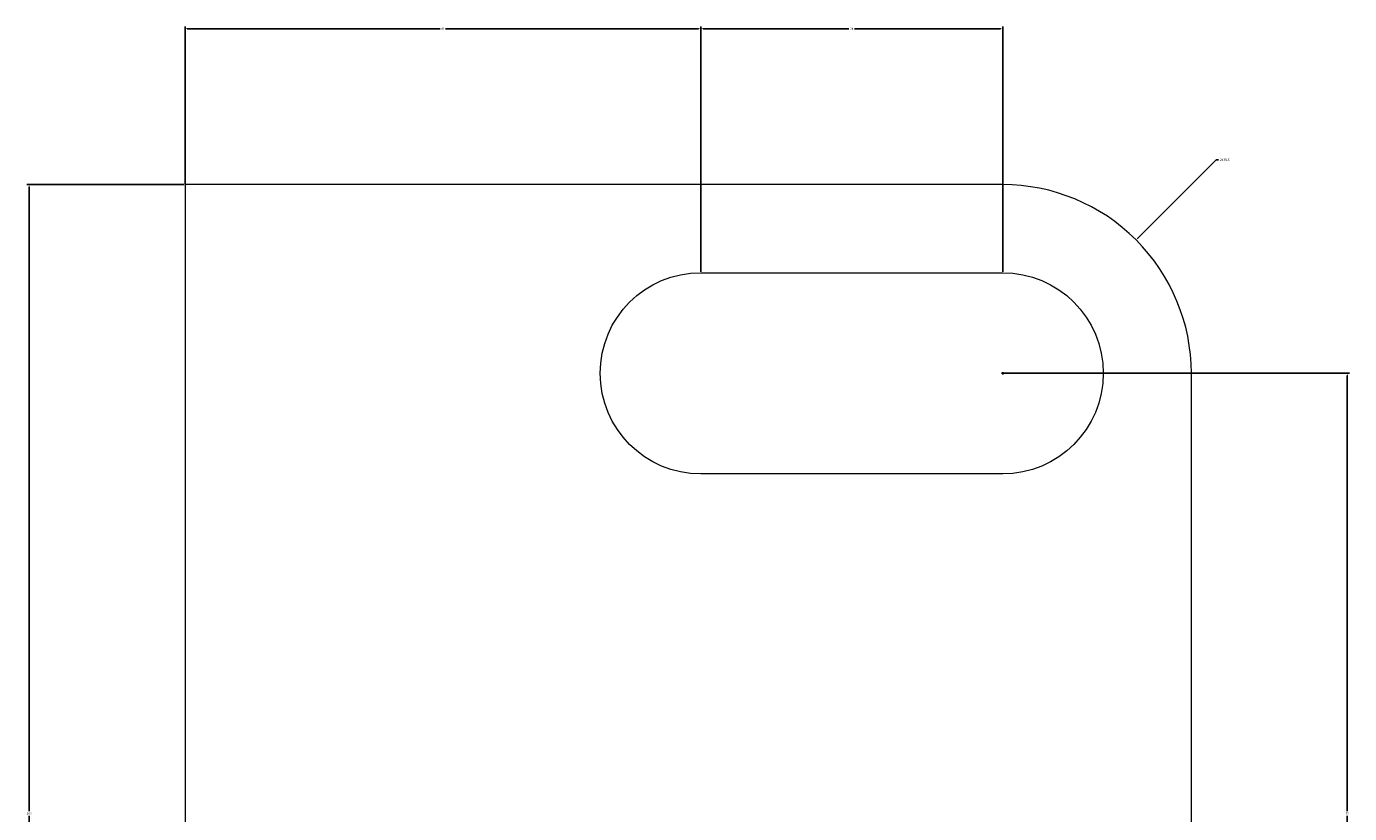
# Model space of a CAD drawing. Units: millimetres. Extents: x 2815 to 2920, y 1079 to 1204.
# Tile 2 of 2: x 2815 to 2920, y 1141 to 1204. Entities that reach past the tile are written whole.
import ezdxf

# ---------------------------------------------------------------- set-up
doc = ezdxf.new("R2010")
doc.units = ezdxf.units.MM
doc.layers.add('M-CONS', color=7, linetype='Continuous', lineweight=18)
doc.layers.add('M-DIMS', color=2, linetype='Continuous', lineweight=18)
doc.styles.get("Standard").update_dxf_attribs({"font": 'arial.ttf'})
doc.dimstyles.get("Standard").update_dxf_attribs({"dimtxt": 0.18, "dimasz": 0.18, "dimexe": 0.18, "dimexo": 0.0625, "dimgap": 0.09, "dimtad": 0, "dimtih": 1, "dimtoh": 1, "dimdec": 4, "dimzin": 0, "dimdsep": 46, "dimtxsty": 'Standard', "dimcen": 0.09, "dimadec": 0, "dimazin": 0, "dimtfac": 1, "dimtdec": 4, "dimtofl": 0, "dimtmove": 0, "dimatfit": 3, "dimfxl": 1, "dimtolj": 1, "dimtzin": 0, "dimarcsym": 0})

# ---------------------------------------------------------------- blocks, each defined once
blk = doc.blocks.new('*D2')
at = {"layer": 'Defpoints', "color": 0, "transparency": 16777216}
for p in [(2815.05, 1191.18), (2827.45, 1191.18), (2827.45, 1091.18)]:
    blk.add_point(p, dxfattribs=at)
at = {"layer": 'M-DIMS', "color": 0, "lineweight": -2, "transparency": 16777216}
for p, q in [((2827.38, 1191.18), (2814.87, 1191.18)), ((2815.05, 1191), (2815.05, 1141.36)), ((2815.05, 1091.36), (2815.05, 1140.99)), ((2827.38, 1091.18), (2814.87, 1091.18))]:
    blk.add_line(p, q, dxfattribs=at)
at = {"layer": 'M-DIMS', "color": 0, "transparency": 16777216}
for points in [[(2815.02, 1191), (2815.08, 1191), (2815.05, 1191.18)], [(2815.02, 1091.36), (2815.08, 1091.36), (2815.05, 1091.18)]]:
    blk.add_solid(points, dxfattribs=at)
at = {"layer": 'M-DIMS', "color": 0, "transparency": 16777216, "insert": (2815.05, 1141.18), "char_height": 0.18, "attachment_point": 5}
blk.add_mtext('\\A1;100', dxfattribs=at)
blk = doc.blocks.new('*D3')
at = {"layer": 'Defpoints', "color": 0, "transparency": 16777216}
for p in [(2868.45, 1203.58), (2827.45, 1191.18), (2868.45, 1184.18)]:
    blk.add_point(p, dxfattribs=at)
at = {"layer": 'M-DIMS', "color": 0, "lineweight": -2, "transparency": 16777216}
for p, q in [((2827.45, 1191.24), (2827.45, 1203.76)), ((2827.63, 1203.58), (2847.74, 1203.58)), ((2868.27, 1203.58), (2848.15, 1203.58)), ((2868.45, 1184.24), (2868.45, 1203.76))]:
    blk.add_line(p, q, dxfattribs=at)
at = {"layer": 'M-DIMS', "color": 0, "transparency": 16777216}
for points in [[(2827.63, 1203.61), (2827.63, 1203.55), (2827.45, 1203.58)], [(2868.27, 1203.61), (2868.27, 1203.55), (2868.45, 1203.58)]]:
    blk.add_solid(points, dxfattribs=at)
at = {"layer": 'M-DIMS', "color": 0, "transparency": 16777216, "insert": (2847.95, 1203.58), "char_height": 0.18, "attachment_point": 5}
blk.add_mtext('\\A1;41', dxfattribs=at)
blk = doc.blocks.new('*D4')
at = {"layer": 'Defpoints', "color": 0, "transparency": 16777216}
for p in [(2892.45, 1203.58), (2868.45, 1184.18), (2892.45, 1184.18)]:
    blk.add_point(p, dxfattribs=at)
at = {"layer": 'M-DIMS', "color": 0, "lineweight": -2, "transparency": 16777216}
for p, q in [((2868.45, 1184.24), (2868.45, 1203.76)), ((2868.63, 1203.58), (2880.23, 1203.58)), ((2892.27, 1203.58), (2880.67, 1203.58)), ((2892.45, 1184.24), (2892.45, 1203.76))]:
    blk.add_line(p, q, dxfattribs=at)
at = {"layer": 'M-DIMS', "color": 0, "transparency": 16777216}
for points in [[(2868.63, 1203.61), (2868.63, 1203.55), (2868.45, 1203.58)], [(2892.27, 1203.61), (2892.27, 1203.55), (2892.45, 1203.58)]]:
    blk.add_solid(points, dxfattribs=at)
at = {"layer": 'M-DIMS', "color": 0, "transparency": 16777216, "insert": (2880.45, 1203.58), "char_height": 0.18, "attachment_point": 5}
blk.add_mtext('\\A1;24', dxfattribs=at)
blk = doc.blocks.new('*D6')
at = {"layer": 'Defpoints', "color": 0, "transparency": 16777216}
for p in [(2892.45, 1176.18), (2919.85, 1176.18), (2892.45, 1106.18)]:
    blk.add_point(p, dxfattribs=at)
at = {"layer": 'M-DIMS', "color": 0, "lineweight": -2, "transparency": 16777216}
for p, q in [((2892.51, 1176.18), (2920.03, 1176.18)), ((2919.85, 1176), (2919.85, 1141.36)), ((2919.85, 1106.36), (2919.85, 1140.99)), ((2892.51, 1106.18), (2920.03, 1106.18))]:
    blk.add_line(p, q, dxfattribs=at)
at = {"layer": 'M-DIMS', "color": 0, "transparency": 16777216}
for points in [[(2919.82, 1176), (2919.88, 1176), (2919.85, 1176.18)], [(2919.82, 1106.36), (2919.88, 1106.36), (2919.85, 1106.18)]]:
    blk.add_solid(points, dxfattribs=at)
at = {"layer": 'M-DIMS', "color": 0, "transparency": 16777216, "insert": (2919.85, 1141.18), "char_height": 0.18, "attachment_point": 5}
blk.add_mtext('\\A1;70', dxfattribs=at)
blk = doc.blocks.new('*D7')
at = {"layer": 'Defpoints', "color": 0, "transparency": 16777216}
for p in [(2903.05, 1186.78), (2892.45, 1176.18)]:
    blk.add_point(p, dxfattribs=at)
at = {"layer": 'M-DIMS', "color": 0, "lineweight": -2, "transparency": 16777216}
for p, q in [((2909.42, 1193.15), (2903.18, 1186.91)), ((2909.6, 1193.15), (2909.42, 1193.15)), ((2892.36, 1176.18), (2892.54, 1176.18)), ((2892.45, 1176.09), (2892.45, 1176.27))]:
    blk.add_line(p, q, dxfattribs=at)
at = {"layer": 'M-DIMS', "color": 0, "transparency": 16777216}
blk.add_solid([(2903.16, 1186.93), (2903.2, 1186.89), (2903.05, 1186.78)], dxfattribs=at)
at = {"layer": 'M-DIMS', "color": 0, "transparency": 16777216, "insert": (2910.1, 1193.15), "char_height": 0.18, "attachment_point": 5}
blk.add_mtext('\\A1;2X R15', dxfattribs=at)

msp = doc.modelspace()

# ---------------------------------------------------------------- linework, layer by layer
at = {"layer": 'M-CONS'}
for points in [[(2907.45, 1176.18, 0.414214), (2892.45, 1191.18), (2827.45, 1191.18), (2827.45, 1091.18), (2892.45, 1091.18, 0.414214), (2907.45, 1106.18)], [(2868.45, 1184.18), (2892.45, 1184.18, -1), (2892.45, 1168.18), (2868.45, 1168.18, -1)]]:
    msp.add_lwpolyline(points, format="xyb", close=True, dxfattribs=at)

# ---------------------------------------------------------------- dimensions: what is measured, and where the dimension line sits
at = {"layer": 'M-DIMS'}
for base, p1, p2, picture, middle in [((2868.45, 1203.58), (2827.45, 1191.18), (2868.45, 1184.18), '*D3', (2847.95, 1203.58)), ((2892.45, 1203.58), (2868.45, 1184.18), (2892.45, 1184.18), '*D4', (2880.45, 1203.58))]:
    dim = msp.add_linear_dim(base=base, p1=p1, p2=p2, dimstyle='Standard', override={"dimdec": 0, "dimlfac": 1, "dimrnd": 0, "dimzin": 0, "dimdsep": 46, "dimlunit": 2}, dxfattribs=at)
    dim.commit()
    dim.dimension.update_dxf_attribs({"geometry": picture, "text_midpoint": middle})
dim = msp.add_radius_dim(center=(2892.45, 1176.18), mpoint=(2903.05, 1186.78), text='2X <>', dimstyle='Standard', override={"dimdec": 0, "dimlfac": 1, "dimrnd": 0, "dimzin": 0, "dimdsep": 46, "dimlunit": 2}, dxfattribs=at)
dim.commit()
dim.dimension.update_dxf_attribs({"geometry": '*D7', "text_midpoint": (2910.1, 1193.15), "dimtype": 164})
for base, p1, p2, picture, middle in [((2815.05, 1191.18), (2827.45, 1091.18), (2827.45, 1191.18), '*D2', (2815.05, 1141.18)), ((2919.85, 1176.18), (2892.45, 1106.18), (2892.45, 1176.18), '*D6', (2919.85, 1141.18))]:
    dim = msp.add_linear_dim(base=base, p1=p1, p2=p2, angle=90, dimstyle='Standard', override={"dimdec": 0, "dimlfac": 1, "dimrnd": 0, "dimzin": 0, "dimdsep": 46, "dimlunit": 2}, dxfattribs=at)
    dim.commit()
    dim.dimension.update_dxf_attribs({"geometry": picture, "text_midpoint": middle})

doc.saveas('drawing.dxf')
